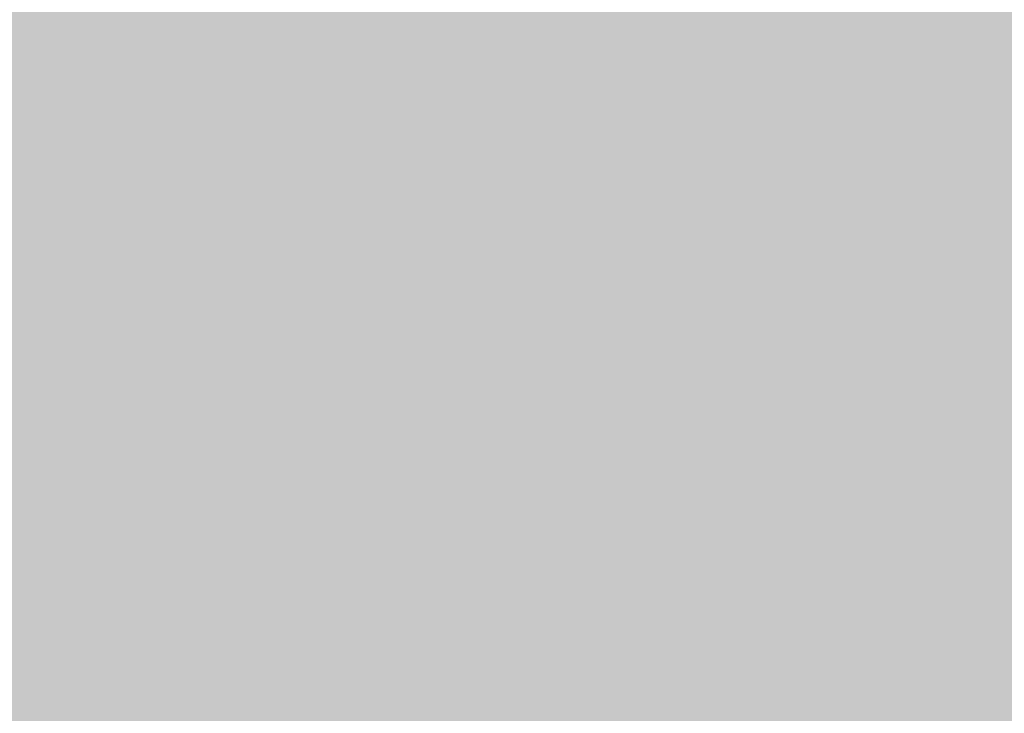
# Model space of a CAD drawing. Units: millimetres. Extents: x -22994 to 29398, y -19990 to 20176.
# Tile 58 of 135: x 216 to 237, y 65 to 80. Entities that reach past the tile are written whole.
import ezdxf
from ezdxf import colors
from ezdxf.entities.mleader import LeaderData, LeaderLine
from ezdxf.math import Vec2, Vec3

# ---------------------------------------------------------------- set-up
doc = ezdxf.new("R2010")
doc.units = ezdxf.units.MM
doc.header["$MEASUREMENT"] = 0
doc.layers.add('M-ANNO-TEXT', color=7, linetype='Continuous', lineweight=25)
doc.layers.add('M-DIMS', color=2, linetype='Continuous', lineweight=18)
doc.styles.get("Standard").update_dxf_attribs({"font": 'arial.ttf'})
doc.dimstyles.get("Standard").update_dxf_attribs({"dimtxt": 0.18, "dimasz": 10000, "dimexe": 0.18, "dimexo": 0.0625, "dimgap": 0.09, "dimtad": 0, "dimtih": 1, "dimtoh": 1, "dimdec": 0, "dimzin": 0, "dimdsep": 46, "dimtxsty": 'Standard', "dimcen": 0.09, "dimadec": 0, "dimazin": 0, "dimtfac": 1, "dimtdec": 0, "dimtofl": 0, "dimtmove": 0, "dimatfit": 3, "dimfxl": 1, "dimtolj": 1, "dimtzin": 0, "dimlwd": 30, "dimarcsym": 0})

# ---------------------------------------------------------------- blocks, each defined once
blk = doc.blocks.new('*D2')
at = {"layer": 'Defpoints', "color": 0, "transparency": 16777216}
for p in [(6.677, 10.271), (290.852, 10.271), (290.852, -5.079)]:
    blk.add_point(p, dxfattribs=at)
at = {"layer": 'M-DIMS', "color": 0, "lineweight": -2, "transparency": 16777216}
for p, q in [((6.677, 10.209), (6.677, -5.259)), ((290.852, 10.209), (290.852, -5.259))]:
    blk.add_line(p, q, dxfattribs=at)
at = {"layer": 'M-DIMS', "color": 0, "lineweight": 30, "transparency": 16777216}
for p, q in [((-9993.323, -5.079), (-19993.323, -5.079)), ((10290.852, -5.079), (20290.852, -5.079))]:
    blk.add_line(p, q, dxfattribs=at)
at = {"layer": 'M-DIMS', "color": 0, "transparency": 16777216}
for points in [[(-9993.323, 1661.588), (-9993.323, -1671.745), (6.677, -5.079)], [(10290.852, 1661.588), (10290.852, -1671.745), (290.852, -5.079)]]:
    blk.add_solid(points, dxfattribs=at)
at = {"layer": 'M-DIMS', "color": 0, "transparency": 16777216, "insert": (148.765, -5.079), "char_height": 0.18, "attachment_point": 5}
blk.add_mtext('\\A1;284.2', dxfattribs=at)
blk = doc.blocks.new('*D3')
at = {"layer": 'Defpoints', "color": 0, "transparency": 16777216}
for p in [(110.265, 204.165), (110.265, 176.366), (95.833, 127.967)]:
    blk.add_point(p, dxfattribs=at)
at = {"layer": 'M-DIMS', "color": 0, "lineweight": -2, "transparency": 16777216}
for p, q in [((95.833, 128.03), (95.833, 204.345)), ((110.265, 176.429), (110.265, 204.345))]:
    blk.add_line(p, q, dxfattribs=at)
at = {"layer": 'M-DIMS', "color": 0, "lineweight": 30, "transparency": 16777216}
for p, q in [((-9904.167, 204.165), (-19904.167, 204.165)), ((10110.265, 204.165), (20110.265, 204.165))]:
    blk.add_line(p, q, dxfattribs=at)
at = {"layer": 'M-DIMS', "color": 0, "transparency": 16777216}
for points in [[(-9904.167, 1870.832), (-9904.167, -1462.501), (95.833, 204.165)], [(10110.265, 1870.832), (10110.265, -1462.501), (110.265, 204.165)]]:
    blk.add_solid(points, dxfattribs=at)
at = {"layer": 'M-DIMS', "color": 0, "transparency": 16777216, "insert": (103.049, 204.165), "char_height": 0.18, "attachment_point": 5}
blk.add_mtext('\\A1;14.432', dxfattribs=at)
blk = doc.blocks.new('*D4')
at = {"layer": 'Defpoints', "color": 0, "transparency": 16777216}
for p in [(116.265, 204.165), (110.265, 176.366), (116.265, 176.366)]:
    blk.add_point(p, dxfattribs=at)
at = {"layer": 'M-DIMS', "color": 0, "lineweight": -2, "transparency": 16777216}
for p, q in [((110.265, 176.429), (110.265, 204.345)), ((116.265, 176.429), (116.265, 204.345))]:
    blk.add_line(p, q, dxfattribs=at)
at = {"layer": 'M-DIMS', "color": 0, "lineweight": 30, "transparency": 16777216}
for p, q in [((-9889.735, 204.165), (-19889.735, 204.165)), ((10116.265, 204.165), (20116.265, 204.165))]:
    blk.add_line(p, q, dxfattribs=at)
at = {"layer": 'M-DIMS', "color": 0, "transparency": 16777216}
for points in [[(-9889.735, 1870.832), (-9889.735, -1462.501), (110.265, 204.165)], [(10116.265, 1870.832), (10116.265, -1462.501), (116.265, 204.165)]]:
    blk.add_solid(points, dxfattribs=at)
at = {"layer": 'M-DIMS', "color": 0, "transparency": 16777216, "insert": (113.265, 204.165), "char_height": 0.18, "attachment_point": 5}
blk.add_mtext('\\A1;6', dxfattribs=at)
blk = doc.blocks.new('*D5')
at = {"layer": 'Defpoints', "color": 0, "transparency": 16777216}
for p in [(181.265, 204.165), (116.265, 176.366), (181.265, 176.366)]:
    blk.add_point(p, dxfattribs=at)
at = {"layer": 'M-DIMS', "color": 0, "lineweight": -2, "transparency": 16777216}
for p, q in [((116.265, 176.429), (116.265, 204.345)), ((181.265, 176.429), (181.265, 204.345))]:
    blk.add_line(p, q, dxfattribs=at)
at = {"layer": 'M-DIMS', "color": 0, "lineweight": 30, "transparency": 16777216}
for p, q in [((-9883.735, 204.165), (-19883.735, 204.165)), ((10181.265, 204.165), (20181.265, 204.165))]:
    blk.add_line(p, q, dxfattribs=at)
at = {"layer": 'M-DIMS', "color": 0, "transparency": 16777216}
for points in [[(-9883.735, 1870.832), (-9883.735, -1462.501), (116.265, 204.165)], [(10181.265, 1870.832), (10181.265, -1462.501), (181.265, 204.165)]]:
    blk.add_solid(points, dxfattribs=at)
at = {"layer": 'M-DIMS', "color": 0, "transparency": 16777216, "insert": (148.765, 204.165), "char_height": 0.18, "attachment_point": 5}
blk.add_mtext('\\A1;65', dxfattribs=at)
blk = doc.blocks.new('*D6')
at = {"layer": 'Defpoints', "color": 0, "transparency": 16777216}
for p in [(187.265, 204.165), (181.265, 176.366), (187.265, 176.366)]:
    blk.add_point(p, dxfattribs=at)
at = {"layer": 'M-DIMS', "color": 0, "lineweight": -2, "transparency": 16777216}
for p, q in [((181.265, 176.429), (181.265, 204.345)), ((187.265, 176.429), (187.265, 204.345))]:
    blk.add_line(p, q, dxfattribs=at)
at = {"layer": 'M-DIMS', "color": 0, "lineweight": 30, "transparency": 16777216}
for p, q in [((-9818.735, 204.165), (-19818.735, 204.165)), ((10187.265, 204.165), (20187.265, 204.165))]:
    blk.add_line(p, q, dxfattribs=at)
at = {"layer": 'M-DIMS', "color": 0, "transparency": 16777216}
for points in [[(-9818.735, 1870.832), (-9818.735, -1462.501), (181.265, 204.165)], [(10187.265, 1870.832), (10187.265, -1462.501), (187.265, 204.165)]]:
    blk.add_solid(points, dxfattribs=at)
at = {"layer": 'M-DIMS', "color": 0, "transparency": 16777216, "insert": (184.265, 204.165), "char_height": 0.18, "attachment_point": 5}
blk.add_mtext('\\A1;6', dxfattribs=at)
blk = doc.blocks.new('*D7')
at = {"layer": 'Defpoints', "color": 0, "transparency": 16777216}
for p in [(201.697, 204.165), (187.265, 176.366), (201.697, 127.967)]:
    blk.add_point(p, dxfattribs=at)
at = {"layer": 'M-DIMS', "color": 0, "lineweight": -2, "transparency": 16777216}
for p, q in [((187.265, 176.429), (187.265, 204.345)), ((201.697, 128.03), (201.697, 204.345))]:
    blk.add_line(p, q, dxfattribs=at)
at = {"layer": 'M-DIMS', "color": 0, "lineweight": 30, "transparency": 16777216}
for p, q in [((-9812.735, 204.165), (-19812.735, 204.165)), ((10201.697, 204.165), (20201.697, 204.165))]:
    blk.add_line(p, q, dxfattribs=at)
at = {"layer": 'M-DIMS', "color": 0, "transparency": 16777216}
for points in [[(-9812.735, 1870.832), (-9812.735, -1462.501), (187.265, 204.165)], [(10201.697, 1870.832), (10201.697, -1462.501), (201.697, 204.165)]]:
    blk.add_solid(points, dxfattribs=at)
at = {"layer": 'M-DIMS', "color": 0, "transparency": 16777216, "insert": (194.481, 204.165), "char_height": 0.18, "attachment_point": 5}
blk.add_mtext('\\A1;14.432', dxfattribs=at)
blk = doc.blocks.new('*D8')
at = {"layer": 'Defpoints', "color": 0, "transparency": 16777216}
for p in [(227.648, 204.165), (227.648, 146.73), (201.697, 127.967)]:
    blk.add_point(p, dxfattribs=at)
at = {"layer": 'M-DIMS', "color": 0, "lineweight": -2, "transparency": 16777216}
for p, q in [((201.697, 128.03), (201.697, 204.345)), ((227.648, 146.792), (227.648, 204.345))]:
    blk.add_line(p, q, dxfattribs=at)
at = {"layer": 'M-DIMS', "color": 0, "lineweight": 30, "transparency": 16777216}
for p, q in [((-9798.303, 204.165), (-19798.303, 204.165)), ((10227.648, 204.165), (20227.648, 204.165))]:
    blk.add_line(p, q, dxfattribs=at)
at = {"layer": 'M-DIMS', "color": 0, "transparency": 16777216}
for points in [[(-9798.303, 1870.832), (-9798.303, -1462.501), (201.697, 204.165)], [(10227.648, 1870.832), (10227.648, -1462.501), (227.648, 204.165)]]:
    blk.add_solid(points, dxfattribs=at)
at = {"layer": 'M-DIMS', "color": 0, "transparency": 16777216, "insert": (214.673, 204.165), "char_height": 0.18, "attachment_point": 5}
blk.add_mtext('\\A1;25.95', dxfattribs=at)
blk = doc.blocks.new('*D9')
at = {"layer": 'Defpoints', "color": 0, "transparency": 16777216}
for p in [(187.265, 176.366), (306.202, 176.366), (290.852, 10.271)]:
    blk.add_point(p, dxfattribs=at)
at = {"layer": 'M-DIMS', "color": 0, "lineweight": 30, "transparency": 16777216}
for p, q in [((306.202, 10176.366), (306.202, 20176.366)), ((306.202, -9989.729), (306.202, -19989.729))]:
    blk.add_line(p, q, dxfattribs=at)
at = {"layer": 'M-DIMS', "color": 0, "lineweight": -2, "transparency": 16777216}
for p, q in [((187.327, 176.366), (306.382, 176.366)), ((290.915, 10.271), (306.382, 10.271))]:
    blk.add_line(p, q, dxfattribs=at)
at = {"layer": 'M-DIMS', "color": 0, "transparency": 16777216}
for points in [[(-1360.465, 10176.366), (1972.869, 10176.366), (306.202, 176.366)], [(-1360.465, -9989.729), (1972.869, -9989.729), (306.202, 10.271)]]:
    blk.add_solid(points, dxfattribs=at)
at = {"layer": 'M-DIMS', "color": 0, "transparency": 16777216, "insert": (306.202, 93.319), "char_height": 0.18, "attachment_point": 5}
blk.add_mtext('\\A1;166.1', dxfattribs=at)
blk = doc.blocks.new('*D10')
at = {"layer": 'Defpoints', "color": 0, "transparency": 16777216}
for p in [(125.65, 136.071), (133.346, 136.071), (133.346, -5.079)]:
    blk.add_point(p, dxfattribs=at)
at = {"layer": 'M-DIMS', "color": 0, "lineweight": -2, "transparency": 16777216}
for p, q in [((125.65, 136.009), (125.65, -5.259)), ((133.346, 136.009), (133.346, -5.259))]:
    blk.add_line(p, q, dxfattribs=at)
at = {"layer": 'M-DIMS', "color": 0, "lineweight": 30, "transparency": 16777216}
for p, q in [((-9874.35, -5.079), (-19874.35, -5.079)), ((10133.346, -5.079), (20133.346, -5.079))]:
    blk.add_line(p, q, dxfattribs=at)
at = {"layer": 'M-DIMS', "color": 0, "transparency": 16777216}
for points in [[(-9874.35, 1661.588), (-9874.35, -1671.745), (125.65, -5.079)], [(10133.346, 1661.588), (10133.346, -1671.745), (133.346, -5.079)]]:
    blk.add_solid(points, dxfattribs=at)
at = {"layer": 'M-DIMS', "color": 0, "transparency": 16777216, "insert": (129.498, -5.079), "char_height": 0.18, "attachment_point": 5}
blk.add_mtext('\\A1;7.696', dxfattribs=at)
blk = doc.blocks.new('*D11')
at = {"layer": 'Defpoints', "color": 0, "transparency": 16777216}
for p in [(133.346, 136.071), (135.65, 136.071), (135.65, -5.079)]:
    blk.add_point(p, dxfattribs=at)
at = {"layer": 'M-DIMS', "color": 0, "lineweight": -2, "transparency": 16777216}
for p, q in [((133.346, 136.009), (133.346, -5.259)), ((135.65, 136.009), (135.65, -5.259))]:
    blk.add_line(p, q, dxfattribs=at)
at = {"layer": 'M-DIMS', "color": 0, "lineweight": 30, "transparency": 16777216}
for p, q in [((-9866.654, -5.079), (-19866.654, -5.079)), ((10135.65, -5.079), (20135.65, -5.079))]:
    blk.add_line(p, q, dxfattribs=at)
at = {"layer": 'M-DIMS', "color": 0, "transparency": 16777216}
for points in [[(-9866.654, 1661.588), (-9866.654, -1671.745), (133.346, -5.079)], [(10135.65, 1661.588), (10135.65, -1671.745), (135.65, -5.079)]]:
    blk.add_solid(points, dxfattribs=at)
at = {"layer": 'M-DIMS', "color": 0, "transparency": 16777216, "insert": (134.498, -5.079), "char_height": 0.18, "attachment_point": 5}
blk.add_mtext('\\A1;2.304', dxfattribs=at)
blk = doc.blocks.new('*D12')
at = {"layer": 'Defpoints', "color": 0, "transparency": 16777216}
for p in [(135.65, 136.071), (145.65, 136.071), (145.65, -5.079)]:
    blk.add_point(p, dxfattribs=at)
at = {"layer": 'M-DIMS', "color": 0, "lineweight": -2, "transparency": 16777216}
for p, q in [((135.65, 136.009), (135.65, -5.259)), ((145.65, 136.009), (145.65, -5.259))]:
    blk.add_line(p, q, dxfattribs=at)
at = {"layer": 'M-DIMS', "color": 0, "lineweight": 30, "transparency": 16777216}
for p, q in [((-9864.35, -5.079), (-19864.35, -5.079)), ((10145.65, -5.079), (20145.65, -5.079))]:
    blk.add_line(p, q, dxfattribs=at)
at = {"layer": 'M-DIMS', "color": 0, "transparency": 16777216}
for points in [[(-9864.35, 1661.588), (-9864.35, -1671.745), (135.65, -5.079)], [(10145.65, 1661.588), (10145.65, -1671.745), (145.65, -5.079)]]:
    blk.add_solid(points, dxfattribs=at)
at = {"layer": 'M-DIMS', "color": 0, "transparency": 16777216, "insert": (140.65, -5.079), "char_height": 0.18, "attachment_point": 5}
blk.add_mtext('\\A1;10', dxfattribs=at)
blk = doc.blocks.new('*D13')
at = {"layer": 'Defpoints', "color": 0, "transparency": 16777216}
for p in [(145.65, 136.071), (155.65, 136.071), (155.65, -5.079)]:
    blk.add_point(p, dxfattribs=at)
at = {"layer": 'M-DIMS', "color": 0, "lineweight": -2, "transparency": 16777216}
for p, q in [((145.65, 136.009), (145.65, -5.259)), ((155.65, 136.009), (155.65, -5.259))]:
    blk.add_line(p, q, dxfattribs=at)
at = {"layer": 'M-DIMS', "color": 0, "lineweight": 30, "transparency": 16777216}
for p, q in [((-9854.35, -5.079), (-19854.35, -5.079)), ((10155.65, -5.079), (20155.65, -5.079))]:
    blk.add_line(p, q, dxfattribs=at)
at = {"layer": 'M-DIMS', "color": 0, "transparency": 16777216}
for points in [[(-9854.35, 1661.588), (-9854.35, -1671.745), (145.65, -5.079)], [(10155.65, 1661.588), (10155.65, -1671.745), (155.65, -5.079)]]:
    blk.add_solid(points, dxfattribs=at)
at = {"layer": 'M-DIMS', "color": 0, "transparency": 16777216, "insert": (150.65, -5.079), "char_height": 0.18, "attachment_point": 5}
blk.add_mtext('\\A1;10', dxfattribs=at)
blk = doc.blocks.new('*D14')
at = {"layer": 'Defpoints', "color": 0, "transparency": 16777216}
for p in [(155.65, 136.071), (165.65, 136.071), (165.65, -5.079)]:
    blk.add_point(p, dxfattribs=at)
at = {"layer": 'M-DIMS', "color": 0, "lineweight": -2, "transparency": 16777216}
for p, q in [((155.65, 136.009), (155.65, -5.259)), ((165.65, 136.009), (165.65, -5.259))]:
    blk.add_line(p, q, dxfattribs=at)
at = {"layer": 'M-DIMS', "color": 0, "lineweight": 30, "transparency": 16777216}
for p, q in [((-9844.35, -5.079), (-19844.35, -5.079)), ((10165.65, -5.079), (20165.65, -5.079))]:
    blk.add_line(p, q, dxfattribs=at)
at = {"layer": 'M-DIMS', "color": 0, "transparency": 16777216}
for points in [[(-9844.35, 1661.588), (-9844.35, -1671.745), (155.65, -5.079)], [(10165.65, 1661.588), (10165.65, -1671.745), (165.65, -5.079)]]:
    blk.add_solid(points, dxfattribs=at)
at = {"layer": 'M-DIMS', "color": 0, "transparency": 16777216, "insert": (160.65, -5.079), "char_height": 0.18, "attachment_point": 5}
blk.add_mtext('\\A1;10', dxfattribs=at)
blk = doc.blocks.new('*D15')
at = {"layer": 'Defpoints', "color": 0, "transparency": 16777216}
for p in [(173.346, 154.788), (173.346, 136.071), (306.202, 136.071)]:
    blk.add_point(p, dxfattribs=at)
at = {"layer": 'M-DIMS', "color": 0, "lineweight": 30, "transparency": 16777216}
for p, q in [((306.202, 10154.788), (306.202, 20154.788)), ((306.202, -9863.929), (306.202, -19863.929))]:
    blk.add_line(p, q, dxfattribs=at)
at = {"layer": 'M-DIMS', "color": 0, "lineweight": -2, "transparency": 16777216}
for p, q in [((173.408, 154.788), (306.382, 154.788)), ((173.408, 136.071), (306.382, 136.071))]:
    blk.add_line(p, q, dxfattribs=at)
at = {"layer": 'M-DIMS', "color": 0, "transparency": 16777216}
for points in [[(-1360.465, 10154.788), (1972.869, 10154.788), (306.202, 154.788)], [(-1360.465, -9863.929), (1972.869, -9863.929), (306.202, 136.071)]]:
    blk.add_solid(points, dxfattribs=at)
at = {"layer": 'M-DIMS', "color": 0, "transparency": 16777216, "insert": (306.202, 145.43), "char_height": 0.18, "attachment_point": 5}
blk.add_mtext('\\A1;18.717', dxfattribs=at)
blk = doc.blocks.new('*D16')
at = {"layer": 'Defpoints', "color": 0, "transparency": 16777216}
for p in [(120.17, 204.165), (110.466, 48.035), (120.17, 48.035)]:
    blk.add_point(p, dxfattribs=at)
at = {"layer": 'M-DIMS', "color": 0, "lineweight": -2, "transparency": 16777216}
for p, q in [((110.466, 48.097), (110.466, 204.345)), ((120.17, 48.097), (120.17, 204.345))]:
    blk.add_line(p, q, dxfattribs=at)
at = {"layer": 'M-DIMS', "color": 0, "lineweight": 30, "transparency": 16777216}
for p, q in [((-9889.534, 204.165), (-19889.534, 204.165)), ((10120.17, 204.165), (20120.17, 204.165))]:
    blk.add_line(p, q, dxfattribs=at)
at = {"layer": 'M-DIMS', "color": 0, "transparency": 16777216}
for points in [[(-9889.534, 1870.832), (-9889.534, -1462.501), (110.466, 204.165)], [(10120.17, 1870.832), (10120.17, -1462.501), (120.17, 204.165)]]:
    blk.add_solid(points, dxfattribs=at)
at = {"layer": 'M-DIMS', "color": 0, "transparency": 16777216, "insert": (115.318, 204.165), "char_height": 0.18, "attachment_point": 5}
blk.add_mtext('\\A1;9.704', dxfattribs=at)
blk = doc.blocks.new('*D17')
at = {"layer": 'Defpoints', "color": 0, "transparency": 16777216}
for p in [(126.17, 204.165), (120.17, 48.035), (126.17, 48.035)]:
    blk.add_point(p, dxfattribs=at)
at = {"layer": 'M-DIMS', "color": 0, "lineweight": -2, "transparency": 16777216}
for p, q in [((120.17, 48.097), (120.17, 204.345)), ((126.17, 48.097), (126.17, 204.345))]:
    blk.add_line(p, q, dxfattribs=at)
at = {"layer": 'M-DIMS', "color": 0, "lineweight": 30, "transparency": 16777216}
for p, q in [((-9879.83, 204.165), (-19879.83, 204.165)), ((10126.17, 204.165), (20126.17, 204.165))]:
    blk.add_line(p, q, dxfattribs=at)
at = {"layer": 'M-DIMS', "color": 0, "transparency": 16777216}
for points in [[(-9879.83, 1870.832), (-9879.83, -1462.501), (120.17, 204.165)], [(10126.17, 1870.832), (10126.17, -1462.501), (126.17, 204.165)]]:
    blk.add_solid(points, dxfattribs=at)
at = {"layer": 'M-DIMS', "color": 0, "transparency": 16777216, "insert": (123.17, 204.165), "char_height": 0.18, "attachment_point": 5}
blk.add_mtext('\\A1;6', dxfattribs=at)
blk = doc.blocks.new('*D18')
at = {"layer": 'Defpoints', "color": 0, "transparency": 16777216}
for p in [(132.17, 204.165), (126.17, 48.035), (132.17, 48.035)]:
    blk.add_point(p, dxfattribs=at)
at = {"layer": 'M-DIMS', "color": 0, "lineweight": -2, "transparency": 16777216}
for p, q in [((126.17, 48.097), (126.17, 204.345)), ((132.17, 48.097), (132.17, 204.345))]:
    blk.add_line(p, q, dxfattribs=at)
at = {"layer": 'M-DIMS', "color": 0, "lineweight": 30, "transparency": 16777216}
for p, q in [((-9873.83, 204.165), (-19873.83, 204.165)), ((10132.17, 204.165), (20132.17, 204.165))]:
    blk.add_line(p, q, dxfattribs=at)
at = {"layer": 'M-DIMS', "color": 0, "transparency": 16777216}
for points in [[(-9873.83, 1870.832), (-9873.83, -1462.501), (126.17, 204.165)], [(10132.17, 1870.832), (10132.17, -1462.501), (132.17, 204.165)]]:
    blk.add_solid(points, dxfattribs=at)
at = {"layer": 'M-DIMS', "color": 0, "transparency": 16777216, "insert": (129.17, 204.165), "char_height": 0.18, "attachment_point": 5}
blk.add_mtext('\\A1;6', dxfattribs=at)
blk = doc.blocks.new('*D19')
at = {"layer": 'Defpoints', "color": 0, "transparency": 16777216}
for p in [(138.17, 204.165), (132.17, 48.035), (138.17, 48.035)]:
    blk.add_point(p, dxfattribs=at)
at = {"layer": 'M-DIMS', "color": 0, "lineweight": -2, "transparency": 16777216}
for p, q in [((132.17, 48.097), (132.17, 204.345)), ((138.17, 48.097), (138.17, 204.345))]:
    blk.add_line(p, q, dxfattribs=at)
at = {"layer": 'M-DIMS', "color": 0, "lineweight": 30, "transparency": 16777216}
for p, q in [((-9867.83, 204.165), (-19867.83, 204.165)), ((10138.17, 204.165), (20138.17, 204.165))]:
    blk.add_line(p, q, dxfattribs=at)
at = {"layer": 'M-DIMS', "color": 0, "transparency": 16777216}
for points in [[(-9867.83, 1870.832), (-9867.83, -1462.501), (132.17, 204.165)], [(10138.17, 1870.832), (10138.17, -1462.501), (138.17, 204.165)]]:
    blk.add_solid(points, dxfattribs=at)
at = {"layer": 'M-DIMS', "color": 0, "transparency": 16777216, "insert": (135.17, 204.165), "char_height": 0.18, "attachment_point": 5}
blk.add_mtext('\\A1;6', dxfattribs=at)
blk = doc.blocks.new('*D20')
at = {"layer": 'Defpoints', "color": 0, "transparency": 16777216}
for p in [(144.17, 204.165), (138.17, 48.035), (144.17, 48.035)]:
    blk.add_point(p, dxfattribs=at)
at = {"layer": 'M-DIMS', "color": 0, "lineweight": -2, "transparency": 16777216}
for p, q in [((138.17, 48.097), (138.17, 204.345)), ((144.17, 48.097), (144.17, 204.345))]:
    blk.add_line(p, q, dxfattribs=at)
at = {"layer": 'M-DIMS', "color": 0, "lineweight": 30, "transparency": 16777216}
for p, q in [((-9861.83, 204.165), (-19861.83, 204.165)), ((10144.17, 204.165), (20144.17, 204.165))]:
    blk.add_line(p, q, dxfattribs=at)
at = {"layer": 'M-DIMS', "color": 0, "transparency": 16777216}
for points in [[(-9861.83, 1870.832), (-9861.83, -1462.501), (138.17, 204.165)], [(10144.17, 1870.832), (10144.17, -1462.501), (144.17, 204.165)]]:
    blk.add_solid(points, dxfattribs=at)
at = {"layer": 'M-DIMS', "color": 0, "transparency": 16777216, "insert": (141.17, 204.165), "char_height": 0.18, "attachment_point": 5}
blk.add_mtext('\\A1;6', dxfattribs=at)
blk = doc.blocks.new('*D21')
at = {"layer": 'Defpoints', "color": 0, "transparency": 16777216}
for p in [(149.116, 204.165), (144.17, 48.035), (149.116, 48.035)]:
    blk.add_point(p, dxfattribs=at)
at = {"layer": 'M-DIMS', "color": 0, "lineweight": -2, "transparency": 16777216}
for p, q in [((144.17, 48.097), (144.17, 204.345)), ((149.116, 48.097), (149.116, 204.345))]:
    blk.add_line(p, q, dxfattribs=at)
at = {"layer": 'M-DIMS', "color": 0, "lineweight": 30, "transparency": 16777216}
for p, q in [((-9855.83, 204.165), (-19855.83, 204.165)), ((10149.116, 204.165), (20149.116, 204.165))]:
    blk.add_line(p, q, dxfattribs=at)
at = {"layer": 'M-DIMS', "color": 0, "transparency": 16777216}
for points in [[(-9855.83, 1870.832), (-9855.83, -1462.501), (144.17, 204.165)], [(10149.116, 1870.832), (10149.116, -1462.501), (149.116, 204.165)]]:
    blk.add_solid(points, dxfattribs=at)
at = {"layer": 'M-DIMS', "color": 0, "transparency": 16777216, "insert": (146.643, 204.165), "char_height": 0.18, "attachment_point": 5}
blk.add_mtext('\\A1;4.945', dxfattribs=at)
blk = doc.blocks.new('*D22')
at = {"layer": 'Defpoints', "color": 0, "transparency": 16777216}
for p in [(149.116, 30.99), (155.116, 30.99), (155.116, -5.079)]:
    blk.add_point(p, dxfattribs=at)
at = {"layer": 'M-DIMS', "color": 0, "lineweight": -2, "transparency": 16777216}
for p, q in [((149.116, 30.927), (149.116, -5.259)), ((155.116, 30.927), (155.116, -5.259))]:
    blk.add_line(p, q, dxfattribs=at)
at = {"layer": 'M-DIMS', "color": 0, "lineweight": 30, "transparency": 16777216}
for p, q in [((-9850.884, -5.079), (-19850.884, -5.079)), ((10155.116, -5.079), (20155.116, -5.079))]:
    blk.add_line(p, q, dxfattribs=at)
at = {"layer": 'M-DIMS', "color": 0, "transparency": 16777216}
for points in [[(-9850.884, 1661.588), (-9850.884, -1671.745), (149.116, -5.079)], [(10155.116, 1661.588), (10155.116, -1671.745), (155.116, -5.079)]]:
    blk.add_solid(points, dxfattribs=at)
at = {"layer": 'M-DIMS', "color": 0, "transparency": 16777216, "insert": (152.116, -5.079), "char_height": 0.18, "attachment_point": 5}
blk.add_mtext('\\A1;6', dxfattribs=at)
blk = doc.blocks.new('*D23')
at = {"layer": 'Defpoints', "color": 0, "transparency": 16777216}
for p in [(155.116, 30.99), (161.116, 30.99), (161.116, -5.079)]:
    blk.add_point(p, dxfattribs=at)
at = {"layer": 'M-DIMS', "color": 0, "lineweight": -2, "transparency": 16777216}
for p, q in [((155.116, 30.927), (155.116, -5.259)), ((161.116, 30.927), (161.116, -5.259))]:
    blk.add_line(p, q, dxfattribs=at)
at = {"layer": 'M-DIMS', "color": 0, "lineweight": 30, "transparency": 16777216}
for p, q in [((-9844.884, -5.079), (-19844.884, -5.079)), ((10161.116, -5.079), (20161.116, -5.079))]:
    blk.add_line(p, q, dxfattribs=at)
at = {"layer": 'M-DIMS', "color": 0, "transparency": 16777216}
for points in [[(-9844.884, 1661.588), (-9844.884, -1671.745), (155.116, -5.079)], [(10161.116, 1661.588), (10161.116, -1671.745), (161.116, -5.079)]]:
    blk.add_solid(points, dxfattribs=at)
at = {"layer": 'M-DIMS', "color": 0, "transparency": 16777216, "insert": (158.116, -5.079), "char_height": 0.18, "attachment_point": 5}
blk.add_mtext('\\A1;6', dxfattribs=at)
blk = doc.blocks.new('*D24')
at = {"layer": 'Defpoints', "color": 0, "transparency": 16777216}
for p in [(161.116, 30.99), (166.439, 30.99), (166.439, -5.079)]:
    blk.add_point(p, dxfattribs=at)
at = {"layer": 'M-DIMS', "color": 0, "lineweight": -2, "transparency": 16777216}
for p, q in [((161.116, 30.927), (161.116, -5.259)), ((166.439, 30.927), (166.439, -5.259))]:
    blk.add_line(p, q, dxfattribs=at)
at = {"layer": 'M-DIMS', "color": 0, "lineweight": 30, "transparency": 16777216}
for p, q in [((-9838.884, -5.079), (-19838.884, -5.079)), ((10166.439, -5.079), (20166.439, -5.079))]:
    blk.add_line(p, q, dxfattribs=at)
at = {"layer": 'M-DIMS', "color": 0, "transparency": 16777216}
for points in [[(-9838.884, 1661.588), (-9838.884, -1671.745), (161.116, -5.079)], [(10166.439, 1661.588), (10166.439, -1671.745), (166.439, -5.079)]]:
    blk.add_solid(points, dxfattribs=at)
at = {"layer": 'M-DIMS', "color": 0, "transparency": 16777216, "insert": (163.777, -5.079), "char_height": 0.18, "attachment_point": 5}
blk.add_mtext('\\A1;5.323', dxfattribs=at)
blk = doc.blocks.new('*D25')
at = {"layer": 'Defpoints', "color": 0, "transparency": 16777216}
for p in [(166.439, 30.99), (172.439, 30.99), (172.439, -5.079)]:
    blk.add_point(p, dxfattribs=at)
at = {"layer": 'M-DIMS', "color": 0, "lineweight": -2, "transparency": 16777216}
for p, q in [((166.439, 30.927), (166.439, -5.259)), ((172.439, 30.927), (172.439, -5.259))]:
    blk.add_line(p, q, dxfattribs=at)
at = {"layer": 'M-DIMS', "color": 0, "lineweight": 30, "transparency": 16777216}
for p, q in [((-9833.561, -5.079), (-19833.561, -5.079)), ((10172.439, -5.079), (20172.439, -5.079))]:
    blk.add_line(p, q, dxfattribs=at)
at = {"layer": 'M-DIMS', "color": 0, "transparency": 16777216}
for points in [[(-9833.561, 1661.588), (-9833.561, -1671.745), (166.439, -5.079)], [(10172.439, 1661.588), (10172.439, -1671.745), (172.439, -5.079)]]:
    blk.add_solid(points, dxfattribs=at)
at = {"layer": 'M-DIMS', "color": 0, "transparency": 16777216, "insert": (169.439, -5.079), "char_height": 0.18, "attachment_point": 5}
blk.add_mtext('\\A1;6', dxfattribs=at)
blk = doc.blocks.new('*D26')
at = {"layer": 'Defpoints', "color": 0, "transparency": 16777216}
for p in [(172.439, 30.99), (178.439, 30.99), (178.439, -5.079)]:
    blk.add_point(p, dxfattribs=at)
at = {"layer": 'M-DIMS', "color": 0, "lineweight": -2, "transparency": 16777216}
for p, q in [((172.439, 30.927), (172.439, -5.259)), ((178.439, 30.927), (178.439, -5.259))]:
    blk.add_line(p, q, dxfattribs=at)
at = {"layer": 'M-DIMS', "color": 0, "lineweight": 30, "transparency": 16777216}
for p, q in [((-9827.561, -5.079), (-19827.561, -5.079)), ((10178.439, -5.079), (20178.439, -5.079))]:
    blk.add_line(p, q, dxfattribs=at)
at = {"layer": 'M-DIMS', "color": 0, "transparency": 16777216}
for points in [[(-9827.561, 1661.588), (-9827.561, -1671.745), (172.439, -5.079)], [(10178.439, 1661.588), (10178.439, -1671.745), (178.439, -5.079)]]:
    blk.add_solid(points, dxfattribs=at)
at = {"layer": 'M-DIMS', "color": 0, "transparency": 16777216, "insert": (175.439, -5.079), "char_height": 0.18, "attachment_point": 5}
blk.add_mtext('\\A1;6', dxfattribs=at)
blk = doc.blocks.new('*D27')
at = {"layer": 'Defpoints', "color": 0, "transparency": 16777216}
for p in [(178.439, 30.99), (188.117, 30.99), (188.117, -5.079)]:
    blk.add_point(p, dxfattribs=at)
at = {"layer": 'M-DIMS', "color": 0, "lineweight": -2, "transparency": 16777216}
for p, q in [((178.439, 30.927), (178.439, -5.259)), ((188.117, 30.927), (188.117, -5.259))]:
    blk.add_line(p, q, dxfattribs=at)
at = {"layer": 'M-DIMS', "color": 0, "lineweight": 30, "transparency": 16777216}
for p, q in [((-9821.561, -5.079), (-19821.561, -5.079)), ((10188.117, -5.079), (20188.117, -5.079))]:
    blk.add_line(p, q, dxfattribs=at)
at = {"layer": 'M-DIMS', "color": 0, "transparency": 16777216}
for points in [[(-9821.561, 1661.588), (-9821.561, -1671.745), (178.439, -5.079)], [(10188.117, 1661.588), (10188.117, -1671.745), (188.117, -5.079)]]:
    blk.add_solid(points, dxfattribs=at)
at = {"layer": 'M-DIMS', "color": 0, "transparency": 16777216, "insert": (183.278, -5.079), "char_height": 0.18, "attachment_point": 5}
blk.add_mtext('\\A1;9.679', dxfattribs=at)
blk = doc.blocks.new('*D28')
at = {"layer": 'Defpoints', "color": 0, "transparency": 16777216}
for p in [(188.117, 48.035), (306.202, 48.035), (188.117, 30.99)]:
    blk.add_point(p, dxfattribs=at)
at = {"layer": 'M-DIMS', "color": 0, "lineweight": 30, "transparency": 16777216}
for p, q in [((306.202, 10048.035), (306.202, 20048.035)), ((306.202, -9969.01), (306.202, -19969.01))]:
    blk.add_line(p, q, dxfattribs=at)
at = {"layer": 'M-DIMS', "color": 0, "lineweight": -2, "transparency": 16777216}
for p, q in [((188.18, 48.035), (306.382, 48.035)), ((188.18, 30.99), (306.382, 30.99))]:
    blk.add_line(p, q, dxfattribs=at)
at = {"layer": 'M-DIMS', "color": 0, "transparency": 16777216}
for points in [[(-1360.465, 10048.035), (1972.869, 10048.035), (306.202, 48.035)], [(-1360.465, -9969.01), (1972.869, -9969.01), (306.202, 30.99)]]:
    blk.add_solid(points, dxfattribs=at)
at = {"layer": 'M-DIMS', "color": 0, "transparency": 16777216, "insert": (306.202, 39.512), "char_height": 0.18, "attachment_point": 5}
blk.add_mtext('\\A1;17.045', dxfattribs=at)
blk = doc.blocks.new('*D29')
at = {"layer": 'Defpoints', "color": 0, "transparency": 16777216}
for p in [(36.801, 80.045), (64.03, 80.045)]:
    blk.add_point(p, dxfattribs=at)
at = {"layer": 'M-DIMS', "color": 0, "lineweight": -2, "transparency": 16777216}
for p, q in [((50.415, 79.955), (50.415, 80.135)), ((50.325, 80.045), (50.505, 80.045))]:
    blk.add_line(p, q, dxfattribs=at)
at = {"layer": 'M-DIMS', "color": 0, "lineweight": 30, "transparency": 16777216}
blk.add_line((20064.03, 80.03), (10064.03, 80.038), dxfattribs=at)
at = {"layer": 'M-DIMS', "color": 0, "transparency": 16777216}
blk.add_solid([(10064.031, 1746.704), (10064.028, -1586.629), (64.03, 80.045)], dxfattribs=at)
at = {"layer": 'M-DIMS', "color": 0, "transparency": 16777216, "insert": (20064.521, 80.03), "char_height": 0.18, "attachment_point": 5}
blk.add_mtext('\\A1;∅27.23', dxfattribs=at)
blk = doc.blocks.new('*D30')
at = {"layer": 'Defpoints', "color": 0, "transparency": 16777216}
for p in [(216.315, 146.729), (238.982, 146.73)]:
    blk.add_point(p, dxfattribs=at)
at = {"layer": 'M-DIMS', "color": 0, "lineweight": 30, "transparency": 16777216}
blk.add_line((20238.982, 147.496), (10238.982, 147.113), dxfattribs=at)
at = {"layer": 'M-DIMS', "color": 0, "lineweight": -2, "transparency": 16777216}
for p, q in [((227.558, 146.73), (227.738, 146.73)), ((227.648, 146.64), (227.648, 146.82))]:
    blk.add_line(p, q, dxfattribs=at)
at = {"layer": 'M-DIMS', "color": 0, "transparency": 16777216}
blk.add_solid([(10238.918, 1813.78), (10239.046, -1519.554), (238.982, 146.73)], dxfattribs=at)
at = {"layer": 'M-DIMS', "color": 0, "transparency": 16777216, "insert": (20239.544, 147.496), "char_height": 0.18, "attachment_point": 5}
blk.add_mtext('\\A1;∅22.667', dxfattribs=at)
blk = doc.blocks.new('*D31')
at = {"layer": 'Defpoints', "color": 0, "transparency": 16777216}
for p in [(223.164, 146.729), (232.133, 146.73)]:
    blk.add_point(p, dxfattribs=at)
at = {"layer": 'M-DIMS', "color": 0, "lineweight": 30, "transparency": 16777216}
blk.add_line((20232.133, 148.666), (10232.133, 147.698), dxfattribs=at)
at = {"layer": 'M-DIMS', "color": 0, "lineweight": -2, "transparency": 16777216}
for p, q in [((227.558, 146.73), (227.738, 146.73)), ((227.648, 146.64), (227.648, 146.82))]:
    blk.add_line(p, q, dxfattribs=at)
at = {"layer": 'M-DIMS', "color": 0, "transparency": 16777216}
blk.add_solid([(10231.971, 1814.364), (10232.294, -1518.969), (232.133, 146.73)], dxfattribs=at)
at = {"layer": 'M-DIMS', "color": 0, "transparency": 16777216, "insert": (20232.625, 148.666), "char_height": 0.18, "attachment_point": 5}
blk.add_mtext('\\A1;∅8.969', dxfattribs=at)
blk = doc.blocks.new('*D33')
at = {"layer": 'Defpoints', "color": 0, "transparency": 16777216}
for p in [(229.561, 154.377), (232.997, 153.351)]:
    blk.add_point(p, dxfattribs=at)
at = {"layer": 'M-DIMS', "color": 0, "lineweight": -2, "transparency": 16777216}
for p, q in [((229.471, 154.377), (229.651, 154.377)), ((229.561, 154.287), (229.561, 154.467))]:
    blk.add_line(p, q, dxfattribs=at)
at = {"layer": 'M-DIMS', "color": 0, "lineweight": 30, "transparency": 16777216}
for p, q in [((19396.339, -5570.838), (9814.668, -2708.743)), ((29396.339, -5570.838), (19396.339, -5570.838))]:
    blk.add_line(p, q, dxfattribs=at)
at = {"layer": 'M-DIMS', "color": 0, "transparency": 16777216}
blk.add_solid([(10291.684, -1111.798), (9337.652, -4305.689), (232.997, 153.351)], dxfattribs=at)
at = {"layer": 'M-DIMS', "color": 0, "transparency": 16777216, "insert": (29397.012, -5570.838), "char_height": 0.18, "attachment_point": 5}
blk.add_mtext('\\A1;6X R3.586', dxfattribs=at)
blk = doc.blocks.new('*D36')
at = {"layer": 'Defpoints', "color": 0, "transparency": 16777216}
for p in [(46.39, 31.303), (46.387, 26.593)]:
    blk.add_point(p, dxfattribs=at)
at = {"layer": 'M-DIMS', "color": 0, "lineweight": 30, "transparency": 16777216}
for p, q in [((57.15, 20031.301), (51.77, 10031.302)), ((10057.15, 20031.301), (57.15, 20031.301))]:
    blk.add_line(p, q, dxfattribs=at)
at = {"layer": 'M-DIMS', "color": 0, "lineweight": -2, "transparency": 16777216}
for p, q in [((46.299, 28.948), (46.479, 28.948)), ((46.389, 28.858), (46.389, 29.038))]:
    blk.add_line(p, q, dxfattribs=at)
at = {"layer": 'M-DIMS', "color": 0, "transparency": 16777216}
blk.add_solid([(-1614.896, 10032.199), (1718.436, 10030.405), (46.39, 31.303)], dxfattribs=at)
at = {"layer": 'M-DIMS', "color": 0, "transparency": 16777216, "insert": (10057.554, 20031.301), "char_height": 0.18, "attachment_point": 5}
blk.add_mtext('\\A1;∅4.71', dxfattribs=at)
blk = doc.blocks.new('*D37')
at = {"layer": 'Defpoints', "color": 0, "transparency": 16777216}
for p in [(54.834, 118.615), (59.494, 118.614)]:
    blk.add_point(p, dxfattribs=at)
at = {"layer": 'M-DIMS', "color": 0, "lineweight": -2, "transparency": 16777216}
for p, q in [((57.074, 118.614), (57.254, 118.614)), ((57.164, 118.524), (57.164, 118.704))]:
    blk.add_line(p, q, dxfattribs=at)
at = {"layer": 'M-DIMS', "color": 0, "lineweight": 30, "transparency": 16777216}
blk.add_line((20059.493, 116.253), (10059.494, 117.434), dxfattribs=at)
at = {"layer": 'M-DIMS', "color": 0, "transparency": 16777216}
blk.add_solid([(10059.69, 1784.1), (10059.297, -1549.233), (59.494, 118.614)], dxfattribs=at)
at = {"layer": 'M-DIMS', "color": 0, "transparency": 16777216, "insert": (20059.985, 116.253), "char_height": 0.18, "attachment_point": 5}
blk.add_mtext('\\A1;∅4.659', dxfattribs=at)

msp = doc.modelspace()

# ---------------------------------------------------------------- dimensions: what is measured, and where the dimension line sits
at = {"layer": 'M-DIMS'}
for base, p1, p2, override, picture, middle in [((306.202, 176.3662), (290.852, 10.2713), (187.2647, 176.3662), {"dimdec": 1, "dimlfac": 1, "dimrnd": 0, "dimzin": 0, "dimdsep": 46, "dimlunit": 2}, '*D9', (306.202, 93.3187)), ((306.202, 136.0713), (173.3459, 154.788), (173.3459, 136.0713), {"dimdec": 3, "dimlfac": 1, "dimrnd": 0, "dimzin": 0, "dimdsep": 46, "dimlunit": 2}, '*D15', (306.202, 145.4297)), ((306.202, 48.0349), (188.1175, 30.9895), (188.1175, 48.0349), {"dimdec": 3, "dimlfac": 1, "dimrnd": 0, "dimzin": 0, "dimdsep": 46, "dimlunit": 2}, '*D28', (306.202, 39.5122))]:
    dim = msp.add_linear_dim(base=base, p1=p1, p2=p2, angle=90, dimstyle='Standard', override=override, dxfattribs=at)
    dim.commit()
    dim.dimension.update_dxf_attribs({"geometry": picture, "text_midpoint": middle})
for p1, p2, override, picture, middle in [((46.3875, 26.5934), (46.39, 31.3035), {"dimdec": 2, "dimlfac": 1, "dimrnd": 0, "dimzin": 0, "dimdsep": 46, "dimlunit": 2}, '*D36', (10057.5542, 20031.3006)), ((223.1641, 146.7291), (232.1328, 146.73), {"dimdec": 3, "dimlfac": 1, "dimrnd": 0, "dimzin": 0, "dimdsep": 46, "dimlunit": 2}, '*D31', (20232.1327, 148.6656)), ((216.3148, 146.7291), (238.9821, 146.73), {"dimdec": 3, "dimlfac": 1, "dimrnd": 0, "dimzin": 0, "dimdsep": 46, "dimlunit": 2}, '*D30', (20238.9821, 147.4959))]:
    dim = msp.add_diameter_dim_2p(p1=p1, p2=p2, dimstyle='Standard', override=override, dxfattribs=at)
    dim.commit()
    dim.dimension.update_dxf_attribs({"geometry": picture, "text_midpoint": middle, "dimtype": 163})
for base, p1, p2, override, picture, middle in [((110.2647, 204.1654), (95.8327, 127.967), (110.2647, 176.3662), {"dimdec": 3, "dimlfac": 1, "dimrnd": 0, "dimzin": 0, "dimdsep": 46, "dimlunit": 2}, '*D3', (103.0487, 204.1654)), ((116.2647, 204.1654), (110.2647, 176.3662), (116.2647, 176.3662), {"dimdec": 0, "dimlfac": 1, "dimrnd": 0, "dimzin": 0, "dimdsep": 46, "dimlunit": 2}, '*D4', (113.2647, 204.1654)), ((120.1702, 204.1654), (110.4658, 48.0349), (120.1702, 48.0349), {"dimdec": 3, "dimlfac": 1, "dimrnd": 0, "dimzin": 0, "dimdsep": 46, "dimlunit": 2}, '*D16', (115.318, 204.1654)), ((181.2647, 204.1654), (116.2647, 176.3662), (181.2647, 176.3662), {"dimdec": 0, "dimlfac": 1, "dimrnd": 0, "dimzin": 0, "dimdsep": 46, "dimlunit": 2}, '*D5', (148.7647, 204.1654)), ((126.1702, 204.1654), (120.1702, 48.0349), (126.1702, 48.0349), {"dimdec": 0, "dimlfac": 1, "dimrnd": 0, "dimzin": 0, "dimdsep": 46, "dimlunit": 2}, '*D17', (123.1702, 204.1654)), ((132.1702, 204.1654), (126.1702, 48.0349), (132.1702, 48.0349), {"dimdec": 0, "dimlfac": 1, "dimrnd": 0, "dimzin": 0, "dimdsep": 46, "dimlunit": 2}, '*D18', (129.1702, 204.1654)), ((138.1702, 204.1654), (132.1702, 48.0349), (138.1702, 48.0349), {"dimdec": 0, "dimlfac": 1, "dimrnd": 0, "dimzin": 0, "dimdsep": 46, "dimlunit": 2}, '*D19', (135.1702, 204.1654)), ((144.1702, 204.1654), (138.1702, 48.0349), (144.1702, 48.0349), {"dimdec": 0, "dimlfac": 1, "dimrnd": 0, "dimzin": 0, "dimdsep": 46, "dimlunit": 2}, '*D20', (141.1702, 204.1654)), ((149.11567, 204.16539), (144.17023, 48.03494), (149.11567, 48.03494), {"dimdec": 3, "dimlfac": 1, "dimrnd": 0, "dimzin": 0, "dimdsep": 46, "dimlunit": 2}, '*D21', (146.64295, 204.16539)), ((187.2647, 204.1654), (181.2647, 176.3662), (187.2647, 176.3662), {"dimdec": 0, "dimlfac": 1, "dimrnd": 0, "dimzin": 0, "dimdsep": 46, "dimlunit": 2}, '*D6', (184.2647, 204.1654)), ((201.6967, 204.1654), (187.2647, 176.3662), (201.6967, 127.967), {"dimdec": 3, "dimlfac": 1, "dimrnd": 0, "dimzin": 0, "dimdsep": 46, "dimlunit": 2}, '*D7', (194.4807, 204.1654)), ((227.6485, 204.1654), (201.6967, 127.967), (227.6485, 146.7296), {"dimdec": 2, "dimlfac": 1, "dimrnd": 0, "dimzin": 0, "dimdsep": 46, "dimlunit": 2}, '*D8', (214.6726, 204.1654)), ((290.852, -5.0787), (6.6773, 10.2713), (290.852, 10.2713), {"dimdec": 1, "dimlfac": 1, "dimrnd": 0, "dimzin": 0, "dimdsep": 46, "dimlunit": 2}, '*D2', (148.7647, -5.0787)), ((133.3459, -5.0787), (125.6498, 136.0713), (133.3459, 136.0713), {"dimdec": 3, "dimlfac": 1, "dimrnd": 0, "dimzin": 0, "dimdsep": 46, "dimlunit": 2}, '*D10', (129.4978, -5.0787)), ((135.6498, -5.0787), (133.3459, 136.0713), (135.6498, 136.0713), {"dimdec": 3, "dimlfac": 1, "dimrnd": 0, "dimzin": 0, "dimdsep": 46, "dimlunit": 2}, '*D11', (134.4978, -5.0787)), ((145.6498, -5.0787), (135.6498, 136.0713), (145.6498, 136.0713), {"dimdec": 0, "dimlfac": 1, "dimrnd": 0, "dimzin": 0, "dimdsep": 46, "dimlunit": 2}, '*D12', (140.6498, -5.0787)), ((155.6498, -5.0787), (145.6498, 136.0713), (155.6498, 136.0713), {"dimdec": 0, "dimlfac": 1, "dimrnd": 0, "dimzin": 0, "dimdsep": 46, "dimlunit": 2}, '*D13', (150.6498, -5.0787)), ((155.1157, -5.0787), (149.1157, 30.9895), (155.1157, 30.9895), {"dimdec": 0, "dimlfac": 1, "dimrnd": 0, "dimzin": 0, "dimdsep": 46, "dimlunit": 2}, '*D22', (152.1157, -5.0787)), ((161.1157, -5.0787), (155.1157, 30.9895), (161.1157, 30.9895), {"dimdec": 0, "dimlfac": 1, "dimrnd": 0, "dimzin": 0, "dimdsep": 46, "dimlunit": 2}, '*D23', (158.1157, -5.0787)), ((165.6498, -5.0787), (155.6498, 136.0713), (165.6498, 136.0713), {"dimdec": 0, "dimlfac": 1, "dimrnd": 0, "dimzin": 0, "dimdsep": 46, "dimlunit": 2}, '*D14', (160.6498, -5.0787)), ((166.4387, -5.0787), (161.1157, 30.9895), (166.4387, 30.9895), {"dimdec": 3, "dimlfac": 1, "dimrnd": 0, "dimzin": 0, "dimdsep": 46, "dimlunit": 2}, '*D24', (163.7772, -5.0787)), ((172.4387, -5.0787), (166.4387, 30.9895), (172.4387, 30.9895), {"dimdec": 0, "dimlfac": 1, "dimrnd": 0, "dimzin": 0, "dimdsep": 46, "dimlunit": 2}, '*D25', (169.4387, -5.0787)), ((178.4387, -5.0787), (172.4387, 30.9895), (178.4387, 30.9895), {"dimdec": 0, "dimlfac": 1, "dimrnd": 0, "dimzin": 0, "dimdsep": 46, "dimlunit": 2}, '*D26', (175.4387, -5.0787)), ((188.1175, -5.0787), (178.4387, 30.9895), (188.1175, 30.9895), {"dimdec": 3, "dimlfac": 1, "dimrnd": 0, "dimzin": 0, "dimdsep": 46, "dimlunit": 2}, '*D27', (183.2781, -5.0787))]:
    dim = msp.add_linear_dim(base=base, p1=p1, p2=p2, dimstyle='Standard', override=override, dxfattribs=at)
    dim.commit()
    dim.dimension.update_dxf_attribs({"geometry": picture, "text_midpoint": middle})
for p1, p2, override, picture, middle in [((54.8343, 118.6145), (59.4936, 118.614), {"dimdec": 3, "dimlfac": 1, "dimrnd": 0, "dimzin": 0, "dimdsep": 46, "dimlunit": 2}, '*D37', (20059.4934, 116.2531)), ((36.8006, 80.045), (64.0296, 80.045), {"dimdec": 2, "dimlfac": 1, "dimrnd": 0, "dimzin": 0, "dimdsep": 46, "dimlunit": 2}, '*D29', (20064.0296, 80.0303))]:
    dim = msp.add_diameter_dim_2p(p1=p1, p2=p2, dimstyle='Standard', override=override, dxfattribs=at)
    dim.commit()
    dim.dimension.update_dxf_attribs({"geometry": picture, "text_midpoint": middle})
dim = msp.add_radius_dim(center=(229.5613, 154.3773), mpoint=(232.9972, 153.3509), text='6X <>', dimstyle='Standard', override={"dimdec": 3, "dimlfac": 1, "dimrnd": 0, "dimzin": 0, "dimdsep": 46, "dimlunit": 2}, dxfattribs=at)
dim.commit()
dim.dimension.update_dxf_attribs({"geometry": '*D33', "text_midpoint": (29397.0125, -5570.8378)})

# ---------------------------------------------------------------- leaders
at = {"layer": 'M-ANNO-TEXT'}
ml = msp.add_multileader_mtext('Standard', dxfattribs=at)
ml.set_content('combustion chamber', color=256)
ml.set_leader_properties()
ml.build(insert=Vec2(0, 0))
ml.multileader.update_dxf_attribs({"dogleg_length": 0.36, "arrow_head_size": 200})
ctx = ml.context
ctx.base_point, ctx.char_height, ctx.arrow_head_size, ctx.landing_gap_size, ctx.plane_origin = Vec3(215.7321, 57.9149), 3, 200, 0.09, Vec3(189.1175, 57.9149)
notes = []
notes.append((ctx, [(0, (1, 1, 0), (215.3721, 57.9149), (1, 0), 0.36, [(0, [(189.1175, 57.9149)], 0, [])])]))
ctx.mtext.insert, ctx.mtext.flow_direction = Vec3(215.8221, 59.4394), 5
for ctx, leaders in notes:
    for number, flags, end, landing, length, lines in leaders:
        leader = LeaderData()
        leader.index, (leader.has_last_leader_line, leader.has_dogleg_vector, leader.attachment_direction) = number, flags
        leader.last_leader_point, leader.dogleg_vector, leader.dogleg_length = Vec3(end), Vec3(landing), length
        for number, points, colour, breaks in lines:
            line = LeaderLine()
            line.index, line.vertices, line.color, line.breaks = number, Vec3.list(points), colors.encode_raw_color(colour), breaks
            leader.lines.append(line)
        ctx.leaders.append(leader)

doc.saveas('drawing.dxf')
